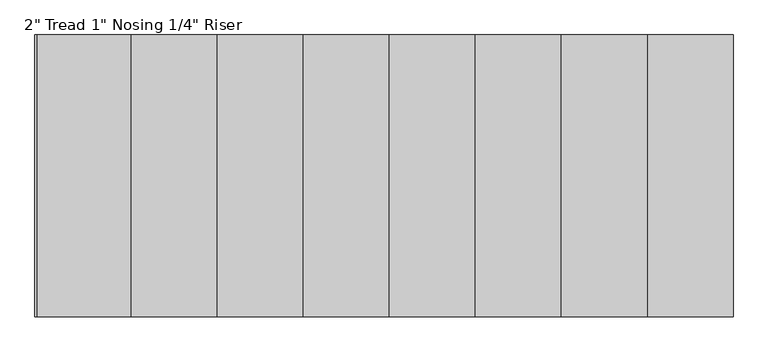
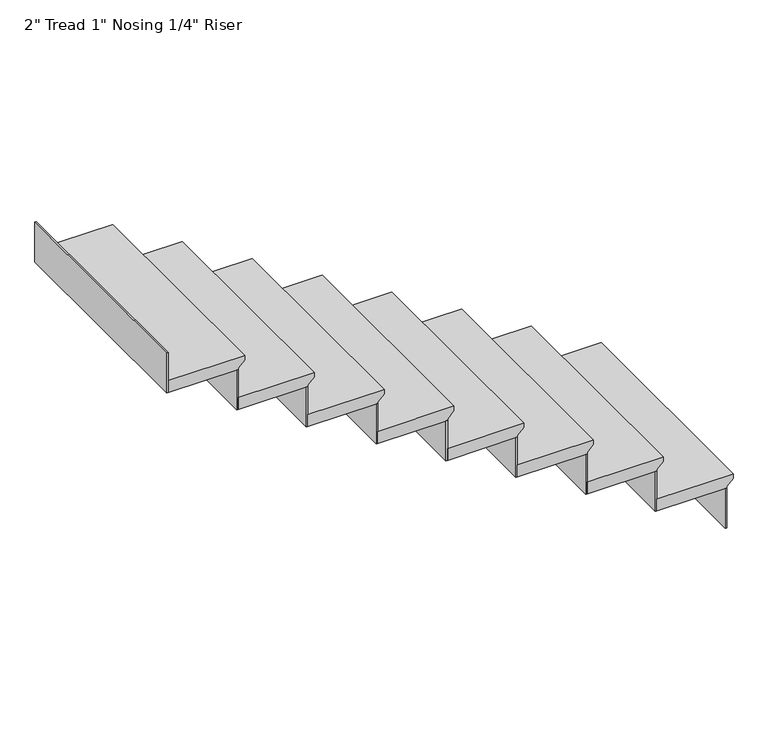
"""IFC4 building model written with IfcOpenShell, lengths in millimetres: stair flight geometry."""

from ifc_helpers import new_model, si_unit, frame, origin, place, context, project, spatial, polyline, outline, extrude, source, transform, mapped, element, save


def stair_flight_d8780985(model_context):
    return source(origin(), model_context, "Body", "SweptSolid", [
        extrude(outline(polyline([(4893.7333333, -2176.9017807), (4893.7333333, -2481.7017807), (4842.9333333, -2481.7017807), (4842.9333333, -2202.3017807), (4849.2833333, -2202.3017807), (4874.6833333, -2176.9017807), (4893.7333333, -2176.9017807)])), frame((0.0, -712.1793133, 0.0), z_axis=(0.0, 1.0, 0.0), x_axis=(0.0, 0.0, 1.0)), (0.0, 0.0, 1.0), 914.4),
        extrude(outline(polyline([(-2208.6517807, 202.2206867), (-2202.3017807, 202.2206867), (-2202.3017807, -712.1793133), (-2208.6517807, -712.1793133), (-2208.6517807, 202.2206867)])), frame((0.0, 0.0, 4673.6), z_axis=(0.0, 0.0, 1.0), x_axis=(1.0, 0.0, 0.0)), (0.0, 0.0, 1.0), 169.3333333),
        extrude(outline(polyline([(-2488.0517807, 202.2206867), (-2481.7017807, 202.2206867), (-2481.7017807, -712.1793133), (-2488.0517807, -712.1793133), (-2488.0517807, 202.2206867)])), frame((0.0, 0.0, 4842.9333333), z_axis=(0.0, 0.0, 1.0), x_axis=(1.0, 0.0, 0.0)), (0.0, 0.0, 1.0), 169.3333333),
        extrude(outline(polyline([(5063.0666667, -2456.3017807), (5063.0666667, -2761.1017807), (5012.2666667, -2761.1017807), (5012.2666667, -2481.7017807), (5018.6166667, -2481.7017807), (5044.0166667, -2456.3017807), (5063.0666667, -2456.3017807)])), frame((0.0, -712.1793133, 0.0), z_axis=(0.0, 1.0, 0.0), x_axis=(0.0, 0.0, 1.0)), (0.0, 0.0, 1.0), 914.4),
        extrude(outline(polyline([(-2767.4517807, 202.2206867), (-2761.1017807, 202.2206867), (-2761.1017807, -712.1793133), (-2767.4517807, -712.1793133), (-2767.4517807, 202.2206867)])), frame((0.0, 0.0, 5012.2666667), z_axis=(0.0, 0.0, 1.0), x_axis=(1.0, 0.0, 0.0)), (0.0, 0.0, 1.0), 169.3333333),
        extrude(outline(polyline([(5232.4, -2735.7017807), (5232.4, -3040.5017807), (5181.6, -3040.5017807), (5181.6, -2761.1017807), (5187.95, -2761.1017807), (5213.35, -2735.7017807), (5232.4, -2735.7017807)])), frame((0.0, -712.1793133, 0.0), z_axis=(0.0, 1.0, 0.0), x_axis=(0.0, 0.0, 1.0)), (0.0, 0.0, 1.0), 914.4),
        extrude(outline(polyline([(-3046.8517807, 202.2206867), (-3040.5017807, 202.2206867), (-3040.5017807, -712.1793133), (-3046.8517807, -712.1793133), (-3046.8517807, 202.2206867)])), frame((0.0, 0.0, 5181.6), z_axis=(0.0, 0.0, 1.0), x_axis=(1.0, 0.0, 0.0)), (0.0, 0.0, 1.0), 169.3333333),
        extrude(outline(polyline([(5401.7333333, -3015.1017807), (5401.7333333, -3319.9017807), (5350.9333333, -3319.9017807), (5350.9333333, -3040.5017807), (5357.2833333, -3040.5017807), (5382.6833333, -3015.1017807), (5401.7333333, -3015.1017807)])), frame((0.0, -712.1793133, 0.0), z_axis=(0.0, 1.0, 0.0), x_axis=(0.0, 0.0, 1.0)), (0.0, 0.0, 1.0), 914.4),
        extrude(outline(polyline([(-3326.2517807, 202.2206867), (-3319.9017807, 202.2206867), (-3319.9017807, -712.1793133), (-3326.2517807, -712.1793133), (-3326.2517807, 202.2206867)])), frame((0.0, 0.0, 5350.9333333), z_axis=(0.0, 0.0, 1.0), x_axis=(1.0, 0.0, 0.0)), (0.0, 0.0, 1.0), 169.3333333),
        extrude(outline(polyline([(5571.0666667, -3294.5017807), (5571.0666667, -3599.3017807), (5520.2666667, -3599.3017807), (5520.2666667, -3319.9017807), (5526.6166667, -3319.9017807), (5552.0166667, -3294.5017807), (5571.0666667, -3294.5017807)])), frame((0.0, -712.1793133, 0.0), z_axis=(0.0, 1.0, 0.0), x_axis=(0.0, 0.0, 1.0)), (0.0, 0.0, 1.0), 914.4),
        extrude(outline(polyline([(-3605.6517807, 202.2206867), (-3599.3017807, 202.2206867), (-3599.3017807, -712.1793133), (-3605.6517807, -712.1793133), (-3605.6517807, 202.2206867)])), frame((0.0, 0.0, 5520.2666667), z_axis=(0.0, 0.0, 1.0), x_axis=(1.0, 0.0, 0.0)), (0.0, 0.0, 1.0), 169.3333333),
        extrude(outline(polyline([(5740.4, -3573.9017807), (5740.4, -3878.7017807), (5689.6, -3878.7017807), (5689.6, -3599.3017807), (5695.95, -3599.3017807), (5721.35, -3573.9017807), (5740.4, -3573.9017807)])), frame((0.0, -712.1793133, 0.0), z_axis=(0.0, 1.0, 0.0), x_axis=(0.0, 0.0, 1.0)), (0.0, 0.0, 1.0), 914.4),
        extrude(outline(polyline([(-3885.0517807, 202.2206867), (-3878.7017807, 202.2206867), (-3878.7017807, -712.1793133), (-3885.0517807, -712.1793133), (-3885.0517807, 202.2206867)])), frame((0.0, 0.0, 5689.6), z_axis=(0.0, 0.0, 1.0), x_axis=(1.0, 0.0, 0.0)), (0.0, 0.0, 1.0), 169.3333333),
        extrude(outline(polyline([(5909.7333333, -3853.3017807), (5909.7333333, -4158.1017807), (5858.9333333, -4158.1017807), (5858.9333333, -3878.7017807), (5865.2833333, -3878.7017807), (5890.6833333, -3853.3017807), (5909.7333333, -3853.3017807)])), frame((0.0, -712.1793133, 0.0), z_axis=(0.0, 1.0, 0.0), x_axis=(0.0, 0.0, 1.0)), (0.0, 0.0, 1.0), 914.4),
        extrude(outline(polyline([(-4164.4517807, 202.2206867), (-4158.1017807, 202.2206867), (-4158.1017807, -712.1793133), (-4164.4517807, -712.1793133), (-4164.4517807, 202.2206867)])), frame((0.0, 0.0, 5858.9333333), z_axis=(0.0, 0.0, 1.0), x_axis=(1.0, 0.0, 0.0)), (0.0, 0.0, 1.0), 169.3333333),
        extrude(outline(polyline([(-4443.8517807, 202.2206867), (-4437.5017807, 202.2206867), (-4437.5017807, -712.1793133), (-4443.8517807, -712.1793133), (-4443.8517807, 202.2206867)])), frame((0.0, 0.0, 6028.2666667), z_axis=(0.0, 0.0, 1.0), x_axis=(1.0, 0.0, 0.0)), (0.0, 0.0, 1.0), 169.3333333),
        extrude(outline(polyline([(6079.0666667, -4132.7017807), (6079.0666667, -4437.5017807), (6028.2666667, -4437.5017807), (6028.2666667, -4158.1017807), (6034.6166667, -4158.1017807), (6060.0166667, -4132.7017807), (6079.0666667, -4132.7017807)])), frame((0.0, -712.1793133, 0.0), z_axis=(0.0, 1.0, 0.0), x_axis=(0.0, 0.0, 1.0)), (0.0, 0.0, 1.0), 914.4),
    ])


if __name__ == "__main__":
    model = new_model("IFC4")
    model_context = context("Model", 3, world=origin())
    ifc_project = project(units=[si_unit("LENGTHUNIT", "METRE", prefix="MILLI")], contexts=[model_context])
    site = spatial("IfcSite", under=ifc_project)
    building = spatial("IfcBuilding", under=site)
    placement = place(None, origin())
    stair_flight_shape = stair_flight_d8780985(model_context)
    element("IfcStairFlight", 1, ObjectType="2\" Tread 1\" Nosing 1/4\" Riser", at=placement, inside=building, context=model_context, shape_type="MappedRepresentation", body=[
        mapped(stair_flight_shape, transform((0.0, 0.0, 0.0), x_axis=(1.0, 0.0, 0.0), y_axis=(0.0, 1.0, 0.0), z_axis=(0.0, 0.0, 1.0))),
    ])
    save(model, "model.ifc")
